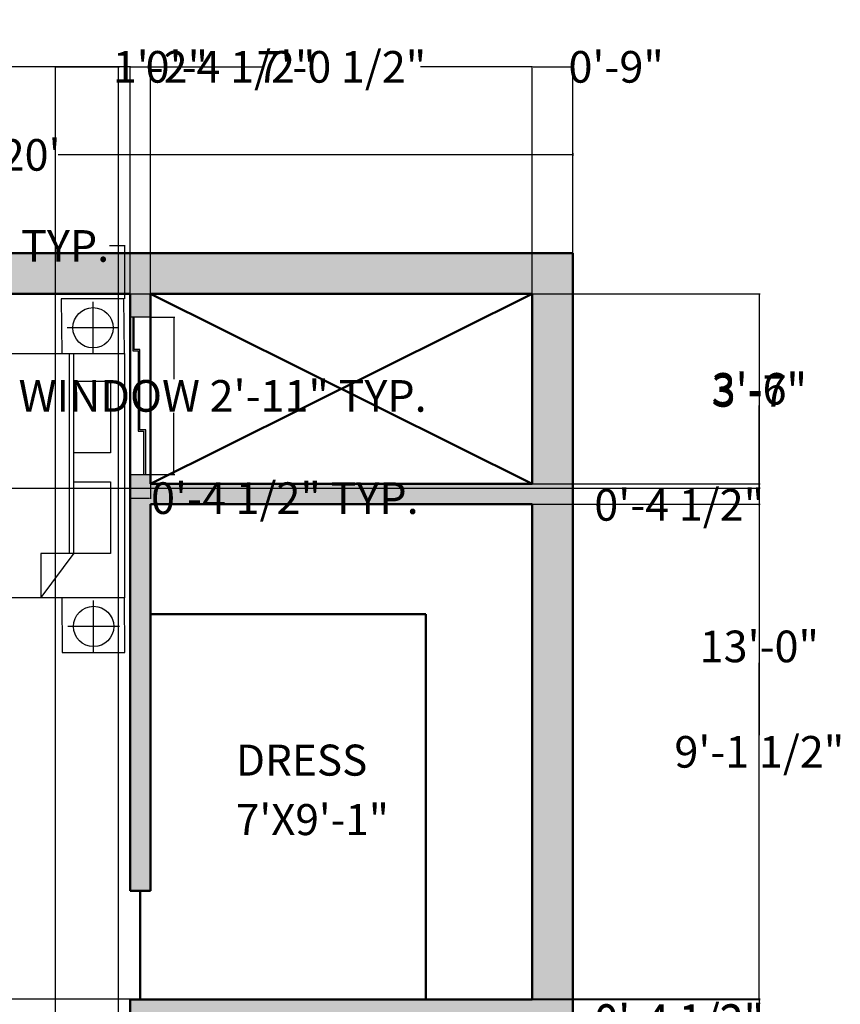
# Model space of a CAD drawing. Units: inches. Extents: x 48 to 822, y -191 to 651.
# Tile 13 of 13: x 626 to 808, y 433 to 651. Entities that reach past the tile are written whole.
import ezdxf

# ---------------------------------------------------------------- set-up
doc = ezdxf.new("R2010")
doc.units = ezdxf.units.IN
doc.header["$MEASUREMENT"] = 0
doc.layers.get('0').update_dxf_attribs({"color": 254})
for name, color, linetype, lineweight in [('A-ANNO-DIMS', 2, 'Continuous', 18), ('A-AREA-IDEN', 7, 'Continuous', 25), ('A-FURN', 8, 'Continuous', 18), ('A-GLAZ', 4, 'Continuous', 25), ('A-WALL', 7, 'Continuous', 50), ('A-WALL-PATT', 8, 'Continuous', 13)]:
    doc.layers.add(name, color=color, linetype=linetype, lineweight=lineweight)
doc.layers.add('furniture', color=250, linetype='Continuous')
doc.styles.get("Standard").update_dxf_attribs({"font": 'arial.ttf'})
doc.dimstyles.get("Standard").update_dxf_attribs({"dimtxt": 7, "dimasz": 0.18, "dimexe": 0.18, "dimexo": 0.0625, "dimgap": 0.09, "dimtad": 0, "dimtih": 1, "dimtoh": 1, "dimzin": 0, "dimdsep": 46, "dimlunit": 3, "dimtxsty": 'Standard', "dimcen": 0.09, "dimadec": 0, "dimazin": 0, "dimtfac": 1, "dimtofl": 0, "dimtmove": 0, "dimatfit": 3, "dimfxl": 1, "dimtolj": 1, "dimtzin": 0, "dimarcsym": 0})

# ---------------------------------------------------------------- blocks, each defined once
blk = doc.blocks.new('CARPET')
at = {"layer": 'furniture'}
for p, q in [((-51.53, -98.11), (-51.53, -55.12)), ((-51.53, -55.12), (-41.27, -55.12)), ((36, -55.12), (51.55, -55.12)), ((51.55, -55.12), (51.55, -98.11)), ((51.55, -98.11), (-51.53, -98.11))]:
    blk.add_line(p, q, dxfattribs=at)
for points, knots in [([(-53.37, -55.99), (-53.22, -55.8), (-52.9, -55.41), (-52.34, -55.8), (-51.89, -56.08), (-51.65, -55.91), (-51.53, -55.83)], [0, 0, 0, 0, 0.653278, 1.290138, 1.740457, 2.114451, 2.114451, 2.114451, 2.114451]), ([(53.37, -55.99), (53.22, -55.8), (52.9, -55.41), (52.34, -55.8), (51.89, -56.08), (51.65, -55.91), (51.53, -55.83)], [0, 0, 0, 0, 0.653278, 1.290138, 1.740457, 2.114451, 2.114451, 2.114451, 2.114451]), ([(-53.37, -57.26), (-53.22, -57.07), (-52.9, -56.67), (-52.34, -57.07), (-51.89, -57.35), (-51.65, -57.17), (-51.53, -57.1)], [0, 0, 0, 0, 0.653278, 1.290138, 1.740457, 2.114451, 2.114451, 2.114451, 2.114451]), ([(-53.37, -58.59), (-53.22, -58.4), (-52.9, -58.01), (-52.34, -58.4), (-51.89, -58.68), (-51.65, -58.5), (-51.53, -58.43)], [0, 0, 0, 0, 0.653278, 1.290138, 1.740457, 2.114451, 2.114451, 2.114451, 2.114451]), ([(53.37, -57.26), (53.22, -57.07), (52.9, -56.67), (52.34, -57.07), (51.89, -57.35), (51.65, -57.17), (51.53, -57.1)], [0, 0, 0, 0, 0.653278, 1.290138, 1.740457, 2.114451, 2.114451, 2.114451, 2.114451]), ([(53.37, -58.59), (53.22, -58.4), (52.9, -58.01), (52.34, -58.4), (51.89, -58.68), (51.65, -58.5), (51.53, -58.43)], [0, 0, 0, 0, 0.653278, 1.290138, 1.740457, 2.114451, 2.114451, 2.114451, 2.114451]), ([(-53.37, -59.78), (-53.22, -59.58), (-52.9, -59.19), (-52.34, -59.58), (-51.89, -59.86), (-51.65, -59.69), (-51.53, -59.61)], [0, 0, 0, 0, 0.653278, 1.290138, 1.740457, 2.114451, 2.114451, 2.114451, 2.114451]), ([(-53.37, -61.22), (-53.22, -61.02), (-52.9, -60.63), (-52.34, -61.02), (-51.89, -61.3), (-51.65, -61.13), (-51.53, -61.05)], [0, 0, 0, 0, 0.653278, 1.290138, 1.740457, 2.114451, 2.114451, 2.114451, 2.114451]), ([(-53.37, -62.44), (-53.22, -62.25), (-52.9, -61.86), (-52.34, -62.25), (-51.89, -62.53), (-51.65, -62.36), (-51.53, -62.28)], [0, 0, 0, 0, 0.653278, 1.290138, 1.740457, 2.114451, 2.114451, 2.114451, 2.114451]), ([(53.37, -59.78), (53.22, -59.58), (52.9, -59.19), (52.34, -59.58), (51.89, -59.86), (51.65, -59.69), (51.53, -59.61)], [0, 0, 0, 0, 0.653278, 1.290138, 1.740457, 2.114451, 2.114451, 2.114451, 2.114451]), ([(53.37, -61.22), (53.22, -61.02), (52.9, -60.63), (52.34, -61.02), (51.89, -61.3), (51.65, -61.13), (51.53, -61.05)], [0, 0, 0, 0, 0.653278, 1.290138, 1.740457, 2.114451, 2.114451, 2.114451, 2.114451]), ([(53.37, -62.44), (53.22, -62.25), (52.9, -61.86), (52.34, -62.25), (51.89, -62.53), (51.65, -62.36), (51.53, -62.28)], [0, 0, 0, 0, 0.653278, 1.290138, 1.740457, 2.114451, 2.114451, 2.114451, 2.114451]), ([(-53.37, -63.63), (-53.22, -63.43), (-52.9, -63.04), (-52.34, -63.43), (-51.89, -63.72), (-51.65, -63.54), (-51.53, -63.46)], [0, 0, 0, 0, 0.653278, 1.290138, 1.740457, 2.114451, 2.114451, 2.114451, 2.114451]), ([(-53.37, -65.07), (-53.22, -64.87), (-52.9, -64.48), (-52.34, -64.87), (-51.89, -65.15), (-51.65, -64.98), (-51.53, -64.9)], [0, 0, 0, 0, 0.653278, 1.290138, 1.740457, 2.114451, 2.114451, 2.114451, 2.114451]), ([(53.37, -63.63), (53.22, -63.43), (52.9, -63.04), (52.34, -63.43), (51.89, -63.72), (51.65, -63.54), (51.53, -63.46)], [0, 0, 0, 0, 0.653278, 1.290138, 1.740457, 2.114451, 2.114451, 2.114451, 2.114451]), ([(53.37, -65.07), (53.22, -64.87), (52.9, -64.48), (52.34, -64.87), (51.89, -65.15), (51.65, -64.98), (51.53, -64.9)], [0, 0, 0, 0, 0.653278, 1.290138, 1.740457, 2.114451, 2.114451, 2.114451, 2.114451]), ([(-53.37, -66.76), (-53.22, -66.56), (-52.9, -66.17), (-52.34, -66.56), (-51.89, -66.84), (-51.65, -66.67), (-51.53, -66.59)], [0, 0, 0, 0, 0.653278, 1.290138, 1.740457, 2.114451, 2.114451, 2.114451, 2.114451]), ([(-53.37, -68.2), (-53.22, -68), (-52.9, -67.61), (-52.34, -68), (-51.89, -68.28), (-51.65, -68.11), (-51.53, -68.03)], [0, 0, 0, 0, 0.653278, 1.290138, 1.740457, 2.114451, 2.114451, 2.114451, 2.114451]), ([(53.37, -66.76), (53.22, -66.56), (52.9, -66.17), (52.34, -66.56), (51.89, -66.84), (51.65, -66.67), (51.53, -66.59)], [0, 0, 0, 0, 0.653278, 1.290138, 1.740457, 2.114451, 2.114451, 2.114451, 2.114451]), ([(53.37, -68.2), (53.22, -68), (52.9, -67.61), (52.34, -68), (51.89, -68.28), (51.65, -68.11), (51.53, -68.03)], [0, 0, 0, 0, 0.653278, 1.290138, 1.740457, 2.114451, 2.114451, 2.114451, 2.114451]), ([(-53.37, -69.53), (-53.22, -69.33), (-52.9, -68.94), (-52.34, -69.33), (-51.89, -69.61), (-51.65, -69.44), (-51.53, -69.36)], [0, 0, 0, 0, 0.653278, 1.290138, 1.740457, 2.114451, 2.114451, 2.114451, 2.114451]), ([(-53.37, -70.79), (-53.22, -70.6), (-52.9, -70.21), (-52.34, -70.6), (-51.89, -70.88), (-51.65, -70.7), (-51.53, -70.63)], [0, 0, 0, 0, 0.653278, 1.290138, 1.740457, 2.114451, 2.114451, 2.114451, 2.114451]), ([(-53.37, -72.12), (-53.22, -71.93), (-52.9, -71.54), (-52.34, -71.93), (-51.89, -72.21), (-51.65, -72.04), (-51.53, -71.96)], [0, 0, 0, 0, 0.653278, 1.290138, 1.740457, 2.114451, 2.114451, 2.114451, 2.114451]), ([(53.37, -69.53), (53.22, -69.33), (52.9, -68.94), (52.34, -69.33), (51.89, -69.61), (51.65, -69.44), (51.53, -69.36)], [0, 0, 0, 0, 0.653278, 1.290138, 1.740457, 2.114451, 2.114451, 2.114451, 2.114451]), ([(53.37, -70.79), (53.22, -70.6), (52.9, -70.21), (52.34, -70.6), (51.89, -70.88), (51.65, -70.7), (51.53, -70.63)], [0, 0, 0, 0, 0.653278, 1.290138, 1.740457, 2.114451, 2.114451, 2.114451, 2.114451]), ([(53.37, -72.12), (53.22, -71.93), (52.9, -71.54), (52.34, -71.93), (51.89, -72.21), (51.65, -72.04), (51.53, -71.96)], [0, 0, 0, 0, 0.653278, 1.290138, 1.740457, 2.114451, 2.114451, 2.114451, 2.114451]), ([(-53.37, -73.31), (-53.22, -73.11), (-52.9, -72.72), (-52.34, -73.11), (-51.89, -73.4), (-51.65, -73.22), (-51.53, -73.14)], [0, 0, 0, 0, 0.653278, 1.290138, 1.740457, 2.114451, 2.114451, 2.114451, 2.114451]), ([(-53.37, -74.75), (-53.22, -74.55), (-52.9, -74.16), (-52.34, -74.55), (-51.89, -74.83), (-51.65, -74.66), (-51.53, -74.58)], [0, 0, 0, 0, 0.653278, 1.290138, 1.740457, 2.114451, 2.114451, 2.114451, 2.114451]), ([(53.37, -73.31), (53.22, -73.11), (52.9, -72.72), (52.34, -73.11), (51.89, -73.4), (51.65, -73.22), (51.53, -73.14)], [0, 0, 0, 0, 0.653278, 1.290138, 1.740457, 2.114451, 2.114451, 2.114451, 2.114451]), ([(53.37, -74.75), (53.22, -74.55), (52.9, -74.16), (52.34, -74.55), (51.89, -74.83), (51.65, -74.66), (51.53, -74.58)], [0, 0, 0, 0, 0.653278, 1.290138, 1.740457, 2.114451, 2.114451, 2.114451, 2.114451]), ([(-53.37, -75.98), (-53.22, -75.78), (-52.9, -75.39), (-52.34, -75.78), (-51.89, -76.06), (-51.65, -75.89), (-51.53, -75.81)], [0, 0, 0, 0, 0.653278, 1.290138, 1.740457, 2.114451, 2.114451, 2.114451, 2.114451]), ([(-53.37, -77.16), (-53.22, -76.96), (-52.9, -76.57), (-52.34, -76.96), (-51.89, -77.25), (-51.65, -77.07), (-51.53, -76.99)], [0, 0, 0, 0, 0.653278, 1.290138, 1.740457, 2.114451, 2.114451, 2.114451, 2.114451]), ([(53.37, -75.98), (53.22, -75.78), (52.9, -75.39), (52.34, -75.78), (51.89, -76.06), (51.65, -75.89), (51.53, -75.81)], [0, 0, 0, 0, 0.653278, 1.290138, 1.740457, 2.114451, 2.114451, 2.114451, 2.114451]), ([(53.37, -77.16), (53.22, -76.96), (52.9, -76.57), (52.34, -76.96), (51.89, -77.25), (51.65, -77.07), (51.53, -76.99)], [0, 0, 0, 0, 0.653278, 1.290138, 1.740457, 2.114451, 2.114451, 2.114451, 2.114451]), ([(-53.37, -78.6), (-53.22, -78.4), (-52.9, -78.01), (-52.34, -78.4), (-51.89, -78.68), (-51.65, -78.51), (-51.53, -78.43)], [0, 0, 0, 0, 0.653278, 1.290138, 1.740457, 2.114451, 2.114451, 2.114451, 2.114451]), ([(-53.37, -80.29), (-53.22, -80.09), (-52.9, -79.7), (-52.34, -80.09), (-51.89, -80.37), (-51.65, -80.2), (-51.53, -80.12)], [0, 0, 0, 0, 0.653278, 1.290138, 1.740457, 2.114451, 2.114451, 2.114451, 2.114451]), ([(53.37, -78.6), (53.22, -78.4), (52.9, -78.01), (52.34, -78.4), (51.89, -78.68), (51.65, -78.51), (51.53, -78.43)], [0, 0, 0, 0, 0.653278, 1.290138, 1.740457, 2.114451, 2.114451, 2.114451, 2.114451]), ([(53.37, -80.29), (53.22, -80.09), (52.9, -79.7), (52.34, -80.09), (51.89, -80.37), (51.65, -80.2), (51.53, -80.12)], [0, 0, 0, 0, 0.653278, 1.290138, 1.740457, 2.114451, 2.114451, 2.114451, 2.114451]), ([(-53.37, -81.73), (-53.22, -81.53), (-52.9, -81.14), (-52.34, -81.53), (-51.89, -81.81), (-51.65, -81.64), (-51.53, -81.56)], [0, 0, 0, 0, 0.653278, 1.290138, 1.740457, 2.114451, 2.114451, 2.114451, 2.114451]), ([(-53.37, -83.06), (-53.22, -82.86), (-52.9, -82.47), (-52.34, -82.86), (-51.89, -83.14), (-51.65, -82.97), (-51.53, -82.89)], [0, 0, 0, 0, 0.653278, 1.290138, 1.740457, 2.114451, 2.114451, 2.114451, 2.114451]), ([(-53.37, -84.18), (-53.22, -83.99), (-52.9, -83.6), (-52.34, -83.99), (-51.89, -84.27), (-51.65, -84.09), (-51.53, -84.02)], [0, 0, 0, 0, 0.653278, 1.290138, 1.740457, 2.114451, 2.114451, 2.114451, 2.114451]), ([(53.37, -81.73), (53.22, -81.53), (52.9, -81.14), (52.34, -81.53), (51.89, -81.81), (51.65, -81.64), (51.53, -81.56)], [0, 0, 0, 0, 0.653278, 1.290138, 1.740457, 2.114451, 2.114451, 2.114451, 2.114451]), ([(53.37, -83.06), (53.22, -82.86), (52.9, -82.47), (52.34, -82.86), (51.89, -83.14), (51.65, -82.97), (51.53, -82.89)], [0, 0, 0, 0, 0.653278, 1.290138, 1.740457, 2.114451, 2.114451, 2.114451, 2.114451]), ([(53.37, -84.18), (53.22, -83.99), (52.9, -83.6), (52.34, -83.99), (51.89, -84.27), (51.65, -84.09), (51.53, -84.02)], [0, 0, 0, 0, 0.653278, 1.290138, 1.740457, 2.114451, 2.114451, 2.114451, 2.114451]), ([(-53.37, -85.51), (-53.22, -85.32), (-52.9, -84.93), (-52.34, -85.32), (-51.89, -85.6), (-51.65, -85.42), (-51.53, -85.35)], [0, 0, 0, 0, 0.653278, 1.290138, 1.740457, 2.114451, 2.114451, 2.114451, 2.114451]), ([(-53.37, -86.7), (-53.22, -86.5), (-52.9, -86.11), (-52.34, -86.5), (-51.89, -86.78), (-51.65, -86.61), (-51.53, -86.53)], [0, 0, 0, 0, 0.653278, 1.290138, 1.740457, 2.114451, 2.114451, 2.114451, 2.114451]), ([(53.37, -85.51), (53.22, -85.32), (52.9, -84.93), (52.34, -85.32), (51.89, -85.6), (51.65, -85.42), (51.53, -85.35)], [0, 0, 0, 0, 0.653278, 1.290138, 1.740457, 2.114451, 2.114451, 2.114451, 2.114451]), ([(53.37, -86.7), (53.22, -86.5), (52.9, -86.11), (52.34, -86.5), (51.89, -86.78), (51.65, -86.61), (51.53, -86.53)], [0, 0, 0, 0, 0.653278, 1.290138, 1.740457, 2.114451, 2.114451, 2.114451, 2.114451]), ([(-53.37, -88.14), (-53.22, -87.94), (-52.9, -87.55), (-52.34, -87.94), (-51.89, -88.22), (-51.65, -88.05), (-51.53, -87.97)], [0, 0, 0, 0, 0.653278, 1.290138, 1.740457, 2.114451, 2.114451, 2.114451, 2.114451]), ([(-53.37, -89.36), (-53.22, -89.17), (-52.9, -88.78), (-52.34, -89.17), (-51.89, -89.45), (-51.65, -89.28), (-51.53, -89.2)], [0, 0, 0, 0, 0.653278, 1.290138, 1.740457, 2.114451, 2.114451, 2.114451, 2.114451]), ([(-53.37, -90.55), (-53.22, -90.35), (-52.9, -89.96), (-52.34, -90.35), (-51.89, -90.64), (-51.65, -90.46), (-51.53, -90.38)], [0, 0, 0, 0, 0.653278, 1.290138, 1.740457, 2.114451, 2.114451, 2.114451, 2.114451]), ([(53.37, -88.14), (53.22, -87.94), (52.9, -87.55), (52.34, -87.94), (51.89, -88.22), (51.65, -88.05), (51.53, -87.97)], [0, 0, 0, 0, 0.653278, 1.290138, 1.740457, 2.114451, 2.114451, 2.114451, 2.114451]), ([(53.37, -89.36), (53.22, -89.17), (52.9, -88.78), (52.34, -89.17), (51.89, -89.45), (51.65, -89.28), (51.53, -89.2)], [0, 0, 0, 0, 0.653278, 1.290138, 1.740457, 2.114451, 2.114451, 2.114451, 2.114451]), ([(53.37, -90.55), (53.22, -90.35), (52.9, -89.96), (52.34, -90.35), (51.9, -90.63), (51.66, -90.47), (51.55, -90.4)], [0, 0, 0, 0, 0.653278, 1.290138, 1.740457, 2.0926, 2.0926, 2.0926, 2.0926]), ([(-53.37, -91.99), (-53.22, -91.79), (-52.9, -91.4), (-52.34, -91.79), (-51.89, -92.07), (-51.65, -91.9), (-51.53, -91.82)], [0, 0, 0, 0, 0.653278, 1.290138, 1.740457, 2.114451, 2.114451, 2.114451, 2.114451]), ([(-53.37, -92.69), (-53.22, -92.48), (-52.9, -92.08), (-52.35, -92.49), (-51.89, -92.77), (-51.65, -92.6), (-51.53, -92.52)], [0, 0, 0, 0, 0.663904, 1.307406, 1.757725, 2.131719, 2.131719, 2.131719, 2.131719]), ([(-53.37, -93.61), (-53.22, -93.42), (-52.9, -93.03), (-52.34, -93.42), (-51.89, -93.7), (-51.65, -93.52), (-51.53, -93.45)], [0, 0, 0, 0, 0.653278, 1.290138, 1.740457, 2.114451, 2.114451, 2.114451, 2.114451]), ([(53.37, -91.99), (53.22, -91.79), (52.9, -91.4), (52.34, -91.79), (51.9, -92.07), (51.66, -91.91), (51.55, -91.83)], [0, 0, 0, 0, 0.653278, 1.290138, 1.740457, 2.0926, 2.0926, 2.0926, 2.0926]), ([(53.37, -92.69), (53.22, -92.49), (52.9, -92.09), (52.34, -92.49), (51.9, -92.77), (51.66, -92.61), (51.55, -92.53)], [0, 0, 0, 0, 0.656792, 1.295826, 1.746145, 2.098292, 2.098292, 2.098292, 2.098292]), ([(53.37, -93.66), (53.22, -93.46), (52.9, -93.07), (52.34, -93.46), (51.9, -93.74), (51.66, -93.58), (51.55, -93.5)], [0, 0, 0, 0, 0.653278, 1.290138, 1.740457, 2.0926, 2.0926, 2.0926, 2.0926]), ([(-53.37, -94.55), (-53.22, -94.35), (-52.9, -93.96), (-52.34, -94.35), (-51.89, -94.63), (-51.65, -94.46), (-51.53, -94.38)], [0, 0, 0, 0, 0.653278, 1.290138, 1.740457, 2.114451, 2.114451, 2.114451, 2.114451]), ([(-53.37, -95.05), (-53.22, -94.85), (-52.9, -94.46), (-52.34, -94.85), (-51.89, -95.14), (-51.65, -94.96), (-51.53, -94.88)], [0, 0, 0, 0, 0.653278, 1.290138, 1.740457, 2.114451, 2.114451, 2.114451, 2.114451]), ([(-53.37, -95.73), (-53.22, -95.54), (-52.9, -95.15), (-52.34, -95.54), (-51.89, -95.82), (-51.65, -95.65), (-51.53, -95.57)], [0, 0, 0, 0, 0.653278, 1.290138, 1.740457, 2.114451, 2.114451, 2.114451, 2.114451]), ([(-53.37, -96.38), (-53.22, -96.18), (-52.9, -95.79), (-52.34, -96.18), (-51.89, -96.47), (-51.65, -96.29), (-51.53, -96.21)], [0, 0, 0, 0, 0.653278, 1.290138, 1.740457, 2.114451, 2.114451, 2.114451, 2.114451]), ([(53.37, -95.78), (53.22, -95.58), (52.9, -95.19), (52.34, -95.58), (51.89, -95.86), (51.65, -95.69), (51.53, -95.61)], [0, 0, 0, 0, 0.653278, 1.290138, 1.740457, 2.114451, 2.114451, 2.114451, 2.114451]), ([(53.37, -96.43), (53.22, -96.23), (52.9, -95.84), (52.34, -96.23), (51.89, -96.51), (51.65, -96.34), (51.53, -96.26)], [0, 0, 0, 0, 0.653278, 1.290138, 1.740457, 2.114451, 2.114451, 2.114451, 2.114451]), ([(53.37, -94.59), (53.22, -94.4), (52.9, -94.01), (52.34, -94.4), (51.9, -94.68), (51.66, -94.51), (51.55, -94.44)], [0, 0, 0, 0, 0.653278, 1.290138, 1.740457, 2.0926, 2.0926, 2.0926, 2.0926]), ([(53.37, -95.1), (53.22, -94.9), (52.9, -94.51), (52.34, -94.9), (51.9, -95.18), (51.66, -95.02), (51.55, -94.94)], [0, 0, 0, 0, 0.653278, 1.290138, 1.740457, 2.0926, 2.0926, 2.0926, 2.0926]), ([(-53.37, -97.17), (-53.22, -96.98), (-52.9, -96.59), (-52.34, -96.98), (-51.89, -97.26), (-51.65, -97.08), (-51.53, -97.01)], [0, 0, 0, 0, 0.653278, 1.290138, 1.740457, 2.114451, 2.114451, 2.114451, 2.114451]), ([(-53.37, -97.99), (-53.22, -97.79), (-52.9, -97.4), (-52.34, -97.79), (-51.89, -98.08), (-51.65, -97.9), (-51.53, -97.82)], [0, 0, 0, 0, 0.653278, 1.290138, 1.740457, 2.114451, 2.114451, 2.114451, 2.114451]), ([(53.37, -97.22), (53.22, -97.02), (52.9, -96.63), (52.34, -97.02), (51.89, -97.3), (51.65, -97.13), (51.53, -97.05)], [0, 0, 0, 0, 0.653278, 1.290138, 1.740457, 2.114451, 2.114451, 2.114451, 2.114451]), ([(53.37, -97.99), (53.22, -97.79), (52.9, -97.4), (52.34, -97.79), (51.89, -98.08), (51.65, -97.9), (51.53, -97.82)], [0, 0, 0, 0, 0.653278, 1.290138, 1.740457, 2.114451, 2.114451, 2.114451, 2.114451])]:
    blk.add_open_spline(points, degree=3, knots=knots, dxfattribs=at)
blk = doc.blocks.new('A$C58D270C6')
at = {"layer": 'furniture'}
for p, q in [((9.09, 124.13), (9.09, 108.87)), ((1.46, 116.5), (16.73, 116.5)), ((14.97, 94.84), (24.62, 107.92)), ((24.62, 94.93), (24.62, 107.92)), ((42.08, 108), (42.08, 36)), ((14.97, 94.93), (24.62, 94.93)), ((14.97, 94.84), (14.97, 36)), ((16.22, 94.93), (16.22, 36)), ((9.25, 36), (9.25, 20.74)), ((1.62, 28.37), (16.88, 28.37))]:
    blk.add_line(p, q, dxfattribs=at)
for points in [[(18.5, 108), (18.34, 124.13), (-0.16, 124.13), (0, 108)], [(0, 108), (77.91, 108), (77.91, 36), (0, 36)], [(4.09, 94.93), (14.97, 94.93), (14.97, 73.83), (4.09, 73.83)], [(4.09, 65.23), (14.97, 65.23), (14.97, 44.13), (4.09, 44.13)], [(18.65, 19.87), (18.5, 36), (0, 36), (0.16, 19.87)]]:
    blk.add_lwpolyline(points, close=True, dxfattribs=at)
for centre in [(9.09, 116.5), (9.25, 28.37)]:
    blk.add_circle(centre, 5.95, dxfattribs=at)
at = {"layer": 'furniture', "xscale": 0.9312884925094044, "yscale": 0.9312884925094044, "zscale": 0.9312884925094044, "rotation": 90}
blk.add_blockref('CARPET', (3.79, 74.47), dxfattribs=at)
blk = doc.blocks.new('*D18')
at = {"layer": 'A-ANNO-DIMS', "color": 0, "lineweight": -2, "transparency": 16777216}
for p, q in [((508.61, 621.85), (508.61, 621.28)), ((508.79, 621.46), (622.52, 621.46)), ((748.43, 621.46), (634.7, 621.46)), ((748.61, 621.85), (748.61, 621.28))]:
    blk.add_line(p, q, dxfattribs=at)
at = {"layer": 'A-ANNO-DIMS', "color": 0, "transparency": 16777216}
for points in [[(508.79, 621.49), (508.79, 621.43), (508.61, 621.46)], [(748.43, 621.49), (748.43, 621.43), (748.61, 621.46)]]:
    blk.add_solid(points, dxfattribs=at)
at = {"layer": 'Defpoints', "color": 0, "transparency": 16777216}
for p in [(508.61, 621.91), (748.61, 621.91), (748.61, 621.46)]:
    blk.add_point(p, dxfattribs=at)
at = {"layer": 'A-ANNO-DIMS', "color": 0, "transparency": 16777216, "insert": (628.61, 621.46), "char_height": 7, "attachment_point": 5}
blk.add_mtext("\\A1;20'", dxfattribs=at)
blk = doc.blocks.new('WIN-900-SLIT')
for p, q in [((271.95, 585.52), (267.45, 585.52)), ((267.45, 585.52), (267.45, 550.72)), ((268.05, 585.52), (268.05, 578.13)), ((268.38, 578.41), (268.38, 585.52)), ((271.95, 550.72), (271.95, 585.52)), ((268.05, 578.13), (269.28, 578.13)), ((269.63, 578.41), (268.38, 578.41)), ((269.28, 578.13), (269.28, 560.35)), ((269.63, 560.61), (269.63, 578.41)), ((269.28, 560.35), (270.46, 560.35)), ((270.92, 560.61), (269.63, 560.61)), ((270.46, 560.35), (270.46, 550.72)), ((270.92, 550.72), (270.92, 560.61)), ((267.45, 550.72), (271.95, 550.72))]:
    blk.add_line(p, q)
blk = doc.blocks.new('*D41')
at = {"layer": 'A-ANNO-DIMS', "color": 0, "lineweight": -2, "transparency": 16777216}
for p, q in [((578, 589.63), (578, 601.49)), ((649.48, 589.63), (649.48, 601.49)), ((578.18, 601.31), (581.44, 601.31)), ((649.3, 601.31), (646.04, 601.31))]:
    blk.add_line(p, q, dxfattribs=at)
at = {"layer": 'A-ANNO-DIMS', "color": 0, "transparency": 16777216}
for points in [[(578.18, 601.34), (578.18, 601.28), (578, 601.31)], [(649.3, 601.34), (649.3, 601.28), (649.48, 601.31)]]:
    blk.add_solid(points, dxfattribs=at)
at = {"layer": 'Defpoints', "color": 0, "transparency": 16777216}
for p in [(578, 601.31), (578, 589.57), (649.48, 589.57)]:
    blk.add_point(p, dxfattribs=at)
at = {"layer": 'A-ANNO-DIMS', "color": 0, "transparency": 16777216, "insert": (613.74, 601.31), "char_height": 7, "attachment_point": 5}
blk.add_mtext('\\A1;5\'-11 1/2" TYP.', dxfattribs=at)
blk = doc.blocks.new('*D50')
at = {"layer": 'A-ANNO-DIMS', "color": 0, "lineweight": -2, "transparency": 16777216}
for p, q in [((655.17, 585.52), (660.51, 585.52)), ((660.33, 585.34), (660.33, 571.83)), ((660.33, 550.9), (660.33, 564.41)), ((655.17, 550.72), (660.51, 550.72))]:
    blk.add_line(p, q, dxfattribs=at)
at = {"layer": 'A-ANNO-DIMS', "color": 0, "transparency": 16777216}
for points in [[(660.3, 585.34), (660.36, 585.34), (660.33, 585.52)], [(660.3, 550.9), (660.36, 550.9), (660.33, 550.72)]]:
    blk.add_solid(points, dxfattribs=at)
at = {"layer": 'Defpoints', "color": 0, "transparency": 16777216}
for p in [(655.11, 585.52), (660.33, 585.52), (655.11, 550.72)]:
    blk.add_point(p, dxfattribs=at)
at = {"layer": 'A-ANNO-DIMS', "color": 0, "transparency": 16777216, "insert": (660.33, 568.12), "char_height": 7, "attachment_point": 5}
blk.add_mtext('\\A1;SLIT WINDOW 2\'-11" TYP.', dxfattribs=at)
blk = doc.blocks.new('*D51')
at = {"layer": 'A-ANNO-DIMS', "color": 0, "lineweight": -2, "transparency": 16777216}
for p, q in [((650.61, 550.66), (650.61, 545.32)), ((655.11, 550.66), (655.11, 545.32)), ((650.79, 545.5), (654.93, 545.5)), ((655.11, 545.5), (655.29, 545.5))]:
    blk.add_line(p, q, dxfattribs=at)
at = {"layer": 'A-ANNO-DIMS', "color": 0, "transparency": 16777216}
for points in [[(650.79, 545.53), (650.79, 545.47), (650.61, 545.5)], [(654.93, 545.53), (654.93, 545.47), (655.11, 545.5)]]:
    blk.add_solid(points, dxfattribs=at)
at = {"layer": 'Defpoints', "color": 0, "transparency": 16777216}
for p in [(650.61, 550.72), (655.11, 550.72), (655.11, 545.5)]:
    blk.add_point(p, dxfattribs=at)
at = {"layer": 'A-ANNO-DIMS', "color": 0, "transparency": 16777216, "insert": (684.87, 545.5), "char_height": 7, "attachment_point": 5}
blk.add_mtext('\\A1;0\'-4 1/2" TYP.', dxfattribs=at)
blk = doc.blocks.new('*D84')
at = {"layer": 'A-ANNO-DIMS', "color": 0, "lineweight": -2, "transparency": 16777216}
for p, q in [((356.51, 590.69), (790.04, 590.69)), ((789.86, 590.51), (789.86, 572.87)), ((789.86, 547.91), (789.86, 565.54)), ((356.51, 547.73), (790.04, 547.73))]:
    blk.add_line(p, q, dxfattribs=at)
at = {"layer": 'A-ANNO-DIMS', "color": 0, "transparency": 16777216}
for points in [[(789.83, 590.51), (789.89, 590.51), (789.86, 590.69)], [(789.83, 547.91), (789.89, 547.91), (789.86, 547.73)]]:
    blk.add_solid(points, dxfattribs=at)
at = {"layer": 'Defpoints', "color": 0, "transparency": 16777216}
for p in [(356.45, 590.69), (356.45, 547.73), (789.86, 547.73)]:
    blk.add_point(p, dxfattribs=at)
at = {"layer": 'A-ANNO-DIMS', "color": 0, "transparency": 16777216, "insert": (789.86, 569.21), "char_height": 7, "attachment_point": 5}
blk.add_mtext('\\A1;3\'-7"', dxfattribs=at)
blk = doc.blocks.new('*D97')
at = {"layer": 'A-ANNO-DIMS', "color": 0, "lineweight": -2, "transparency": 16777216}
for p, q in [((517.61, 590.75), (517.61, 641.12)), ((517.79, 640.94), (572.33, 640.94)), ((650.43, 640.94), (595.89, 640.94)), ((650.61, 590.75), (650.61, 641.12))]:
    blk.add_line(p, q, dxfattribs=at)
at = {"layer": 'A-ANNO-DIMS', "color": 0, "transparency": 16777216}
for points in [[(517.79, 640.97), (517.79, 640.91), (517.61, 640.94)], [(650.43, 640.97), (650.43, 640.91), (650.61, 640.94)]]:
    blk.add_solid(points, dxfattribs=at)
at = {"layer": 'Defpoints', "color": 0, "transparency": 16777216}
for p in [(650.61, 640.94), (517.61, 590.69), (650.61, 590.69)]:
    blk.add_point(p, dxfattribs=at)
at = {"layer": 'A-ANNO-DIMS', "color": 0, "transparency": 16777216, "insert": (584.11, 640.94), "char_height": 7, "attachment_point": 5}
blk.add_mtext('\\A1;11\'-1"', dxfattribs=at)
blk = doc.blocks.new('*D98')
at = {"layer": 'A-ANNO-DIMS', "color": 0, "lineweight": -2, "transparency": 16777216}
for p, q in [((650.61, 590.75), (650.61, 641.12)), ((650.79, 640.94), (654.93, 640.94)), ((655.11, 590.75), (655.11, 641.12)), ((655.11, 640.94), (655.29, 640.94))]:
    blk.add_line(p, q, dxfattribs=at)
at = {"layer": 'A-ANNO-DIMS', "color": 0, "transparency": 16777216}
for points in [[(650.79, 640.97), (650.79, 640.91), (650.61, 640.94)], [(654.93, 640.97), (654.93, 640.91), (655.11, 640.94)]]:
    blk.add_solid(points, dxfattribs=at)
at = {"layer": 'Defpoints', "color": 0, "transparency": 16777216}
for p in [(655.11, 640.94), (650.61, 590.69), (655.11, 590.69)]:
    blk.add_point(p, dxfattribs=at)
at = {"layer": 'A-ANNO-DIMS', "color": 0, "transparency": 16777216, "insert": (672.84, 640.94), "char_height": 7, "attachment_point": 5}
blk.add_mtext('\\A1;0\'-4 1/2"', dxfattribs=at)
blk = doc.blocks.new('*D99')
at = {"layer": 'A-ANNO-DIMS', "color": 0, "lineweight": -2, "transparency": 16777216}
for p, q in [((655.11, 590.75), (655.11, 641.12)), ((655.29, 640.94), (679.84, 640.94)), ((739.43, 640.94), (714.88, 640.94)), ((739.61, 590.75), (739.61, 641.12))]:
    blk.add_line(p, q, dxfattribs=at)
at = {"layer": 'A-ANNO-DIMS', "color": 0, "transparency": 16777216}
for points in [[(655.29, 640.97), (655.29, 640.91), (655.11, 640.94)], [(739.43, 640.97), (739.43, 640.91), (739.61, 640.94)]]:
    blk.add_solid(points, dxfattribs=at)
at = {"layer": 'Defpoints', "color": 0, "transparency": 16777216}
for p in [(739.61, 640.94), (655.11, 590.69), (739.61, 590.69)]:
    blk.add_point(p, dxfattribs=at)
at = {"layer": 'A-ANNO-DIMS', "color": 0, "transparency": 16777216, "insert": (697.36, 640.94), "char_height": 7, "attachment_point": 5}
blk.add_mtext('\\A1;7\'-0 1/2"', dxfattribs=at)
blk = doc.blocks.new('*D100')
at = {"layer": 'A-ANNO-DIMS', "color": 0, "lineweight": -2, "transparency": 16777216}
for p, q in [((739.61, 590.75), (739.61, 641.12)), ((739.79, 640.94), (748.43, 640.94)), ((748.61, 599.75), (748.61, 641.12)), ((748.61, 640.94), (748.79, 640.94))]:
    blk.add_line(p, q, dxfattribs=at)
at = {"layer": 'A-ANNO-DIMS', "color": 0, "transparency": 16777216}
for points in [[(739.79, 640.97), (739.79, 640.91), (739.61, 640.94)], [(748.43, 640.97), (748.43, 640.91), (748.61, 640.94)]]:
    blk.add_solid(points, dxfattribs=at)
at = {"layer": 'Defpoints', "color": 0, "transparency": 16777216}
for p in [(748.61, 640.94), (748.61, 599.69), (739.61, 590.69)]:
    blk.add_point(p, dxfattribs=at)
at = {"layer": 'A-ANNO-DIMS', "color": 0, "transparency": 16777216, "insert": (758.18, 640.94), "char_height": 7, "attachment_point": 5}
blk.add_mtext('\\A1;0\'-9"', dxfattribs=at)
blk = doc.blocks.new('*D105')
at = {"layer": 'A-ANNO-DIMS', "color": 0, "lineweight": -2, "transparency": 16777216}
for p, q in [((517.67, 590.69), (790.04, 590.69)), ((789.86, 590.51), (789.86, 516.35)), ((789.86, 434.87), (789.86, 509.02)), ((517.67, 434.69), (790.04, 434.69))]:
    blk.add_line(p, q, dxfattribs=at)
at = {"layer": 'A-ANNO-DIMS', "color": 0, "transparency": 16777216}
for points in [[(789.83, 590.51), (789.89, 590.51), (789.86, 590.69)], [(789.83, 434.87), (789.89, 434.87), (789.86, 434.69)]]:
    blk.add_solid(points, dxfattribs=at)
at = {"layer": 'Defpoints', "color": 0, "transparency": 16777216}
for p in [(517.61, 590.69), (517.61, 434.69), (789.86, 434.69)]:
    blk.add_point(p, dxfattribs=at)
at = {"layer": 'A-ANNO-DIMS', "color": 0, "transparency": 16777216, "insert": (789.86, 512.69), "char_height": 7, "attachment_point": 5}
blk.add_mtext('\\A1;13\'-0"', dxfattribs=at)
blk = doc.blocks.new('*D106')
at = {"layer": 'A-ANNO-DIMS', "color": 0, "lineweight": -2, "transparency": 16777216}
for p, q in [((517.67, 434.69), (790.04, 434.69)), ((789.86, 434.51), (789.86, 430.37)), ((517.67, 430.19), (790.04, 430.19)), ((789.86, 430.01), (789.68, 430.01)), ((789.86, 430.19), (789.86, 430.01))]:
    blk.add_line(p, q, dxfattribs=at)
at = {"layer": 'A-ANNO-DIMS', "color": 0, "transparency": 16777216}
for points in [[(789.83, 434.51), (789.89, 434.51), (789.86, 434.69)], [(789.83, 430.37), (789.89, 430.37), (789.86, 430.19)]]:
    blk.add_solid(points, dxfattribs=at)
at = {"layer": 'Defpoints', "color": 0, "transparency": 16777216}
for p in [(517.61, 434.69), (517.61, 430.19), (789.86, 430.19)]:
    blk.add_point(p, dxfattribs=at)
at = {"layer": 'A-ANNO-DIMS', "color": 0, "transparency": 16777216, "insert": (772.13, 430.01), "char_height": 7, "attachment_point": 5}
blk.add_mtext('\\A1;0\'-4 1/2"', dxfattribs=at)
blk = doc.blocks.new('*D118')
at = {"layer": 'A-ANNO-DIMS', "color": 0, "lineweight": -2, "transparency": 16777216}
for p, q in [((739.67, 590.69), (790.04, 590.69)), ((789.86, 590.51), (789.86, 573.35)), ((789.86, 548.87), (789.86, 566.02)), ((739.67, 548.69), (790.04, 548.69))]:
    blk.add_line(p, q, dxfattribs=at)
at = {"layer": 'A-ANNO-DIMS', "color": 0, "transparency": 16777216}
for points in [[(789.83, 590.51), (789.89, 590.51), (789.86, 590.69)], [(789.83, 548.87), (789.89, 548.87), (789.86, 548.69)]]:
    blk.add_solid(points, dxfattribs=at)
at = {"layer": 'Defpoints', "color": 0, "transparency": 16777216}
for p in [(739.61, 590.69), (739.61, 548.69), (789.86, 548.69)]:
    blk.add_point(p, dxfattribs=at)
at = {"layer": 'A-ANNO-DIMS', "color": 0, "transparency": 16777216, "insert": (789.86, 569.69), "char_height": 7, "attachment_point": 5}
blk.add_mtext('\\A1;3\'-6"', dxfattribs=at)
blk = doc.blocks.new('*D119')
at = {"layer": 'A-ANNO-DIMS', "color": 0, "lineweight": -2, "transparency": 16777216}
for p, q in [((739.67, 548.69), (790.04, 548.69)), ((789.86, 548.51), (789.86, 544.37)), ((739.67, 544.19), (790.04, 544.19)), ((789.86, 544.01), (789.68, 544.01)), ((789.86, 544.19), (789.86, 544.01))]:
    blk.add_line(p, q, dxfattribs=at)
at = {"layer": 'A-ANNO-DIMS', "color": 0, "transparency": 16777216}
for points in [[(789.83, 548.51), (789.89, 548.51), (789.86, 548.69)], [(789.83, 544.37), (789.89, 544.37), (789.86, 544.19)]]:
    blk.add_solid(points, dxfattribs=at)
at = {"layer": 'Defpoints', "color": 0, "transparency": 16777216}
for p in [(739.61, 548.69), (739.61, 544.19), (789.86, 544.19)]:
    blk.add_point(p, dxfattribs=at)
at = {"layer": 'A-ANNO-DIMS', "color": 0, "transparency": 16777216, "insert": (772.13, 544.01), "char_height": 7, "attachment_point": 5}
blk.add_mtext('\\A1;0\'-4 1/2"', dxfattribs=at)
blk = doc.blocks.new('*D120')
at = {"layer": 'A-ANNO-DIMS', "color": 0, "lineweight": -2, "transparency": 16777216}
for p, q in [((739.67, 544.19), (790.04, 544.19)), ((789.86, 544.01), (789.86, 493.07)), ((789.86, 434.72), (789.86, 485.65)), ((739.67, 434.54), (790.04, 434.54))]:
    blk.add_line(p, q, dxfattribs=at)
at = {"layer": 'A-ANNO-DIMS', "color": 0, "transparency": 16777216}
for points in [[(789.83, 544.01), (789.89, 544.01), (789.86, 544.19)], [(789.83, 434.72), (789.89, 434.72), (789.86, 434.54)]]:
    blk.add_solid(points, dxfattribs=at)
at = {"layer": 'Defpoints', "color": 0, "transparency": 16777216}
for p in [(739.61, 544.19), (739.61, 434.54), (789.86, 434.54)]:
    blk.add_point(p, dxfattribs=at)
at = {"layer": 'A-ANNO-DIMS', "color": 0, "transparency": 16777216, "insert": (789.86, 489.36), "char_height": 7, "attachment_point": 5}
blk.add_mtext('\\A1;9\'-1 1/2"', dxfattribs=at)
blk = doc.blocks.new('*D121')
at = {"layer": 'A-ANNO-DIMS', "color": 0, "lineweight": -2, "transparency": 16777216}
for p, q in [((739.67, 434.54), (790.04, 434.54)), ((789.86, 434.36), (789.86, 430.22)), ((739.67, 430.04), (790.04, 430.04)), ((789.86, 429.86), (789.68, 429.86)), ((789.86, 430.04), (789.86, 429.86))]:
    blk.add_line(p, q, dxfattribs=at)
at = {"layer": 'A-ANNO-DIMS', "color": 0, "transparency": 16777216}
for points in [[(789.83, 434.36), (789.89, 434.36), (789.86, 434.54)], [(789.83, 430.22), (789.89, 430.22), (789.86, 430.04)]]:
    blk.add_solid(points, dxfattribs=at)
at = {"layer": 'Defpoints', "color": 0, "transparency": 16777216}
for p in [(739.61, 434.54), (739.61, 430.04), (789.86, 430.04)]:
    blk.add_point(p, dxfattribs=at)
at = {"layer": 'A-ANNO-DIMS', "color": 0, "transparency": 16777216, "insert": (772.13, 429.86), "char_height": 7, "attachment_point": 5}
blk.add_mtext('\\A1;0\'-4 1/2"', dxfattribs=at)
blk = doc.blocks.new('*D125')
at = {"layer": 'A-ANNO-DIMS', "color": 0, "lineweight": -2, "transparency": 16777216}
for p, q in [((634.1, 295.25), (634.1, 641.12)), ((634.28, 640.94), (647.91, 640.94)), ((648.09, 295.25), (648.09, 641.12)), ((648.09, 640.94), (648.27, 640.94))]:
    blk.add_line(p, q, dxfattribs=at)
at = {"layer": 'A-ANNO-DIMS', "color": 0, "transparency": 16777216}
for points in [[(634.28, 640.97), (634.28, 640.91), (634.1, 640.94)], [(647.91, 640.97), (647.91, 640.91), (648.09, 640.94)]]:
    blk.add_solid(points, dxfattribs=at)
at = {"layer": 'Defpoints', "color": 0, "transparency": 16777216}
for p in [(648.09, 640.94), (634.1, 295.19), (648.09, 295.19)]:
    blk.add_point(p, dxfattribs=at)
at = {"layer": 'A-ANNO-DIMS', "color": 0, "transparency": 16777216, "insert": (657.33, 640.94), "char_height": 7, "attachment_point": 5}
blk.add_mtext('\\A1;1\'-2"', dxfattribs=at)
blk = doc.blocks.new('*D126')
at = {"layer": 'A-ANNO-DIMS', "color": 0, "lineweight": -2, "transparency": 16777216}
for p, q in [((553.61, 295.25), (553.61, 641.12)), ((553.79, 640.94), (580.61, 640.94)), ((647.91, 640.94), (621.09, 640.94)), ((648.09, 295.25), (648.09, 641.12))]:
    blk.add_line(p, q, dxfattribs=at)
at = {"layer": 'A-ANNO-DIMS', "color": 0, "transparency": 16777216}
for points in [[(553.79, 640.97), (553.79, 640.91), (553.61, 640.94)], [(647.91, 640.97), (647.91, 640.91), (648.09, 640.94)]]:
    blk.add_solid(points, dxfattribs=at)
at = {"layer": 'Defpoints', "color": 0, "transparency": 16777216}
for p in [(648.09, 640.94), (553.61, 295.19), (648.09, 295.19)]:
    blk.add_point(p, dxfattribs=at)
at = {"layer": 'A-ANNO-DIMS', "color": 0, "transparency": 16777216, "insert": (600.85, 640.94), "char_height": 7, "attachment_point": 5}
blk.add_mtext('\\A1;7\'-10 1/2"', dxfattribs=at)

msp = doc.modelspace()

# ---------------------------------------------------------------- hatches: boundary and pattern name
at = {"layer": 'A-WALL-PATT'}
h = msp.add_hatch(color=256, dxfattribs=at)
h.dxf.hatch_style = 1
h.paths.add_polyline_path([(614.11, 432.437), (609.61, 432.437), (609.61, 376.187), (535.284, 376.187), (535.284, 371.687), (547.61, 371.687), (547.61, 359.12), (552.11, 359.12), (552.11, 371.687), (609.61, 371.687), (609.61, 335.687), (614.11, 335.687)], flags=17)
h.paths.add_polyline_path([(614.11, 434.687), (609.61, 434.687), (609.61, 432.437), (614.11, 432.437)], flags=17)
h.paths.add_polyline_path([(573.934, 434.687), (517.61, 434.687), (517.61, 590.687), (650.61, 590.687), (650.61, 585.522), (655.11, 585.522), (655.11, 590.687), (739.61, 590.687), (739.61, 548.687), (655.11, 548.687), (655.11, 550.72), (650.61, 550.72), (650.61, 458.608), (655.11, 458.608), (655.11, 544.187), (739.61, 544.187), (739.61, 434.541), (650.61, 434.541), (650.61, 430.041), (739.61, 430.041), (739.61, -16.844), (729.973, -16.844), (729.973, -21.344), (748.61, -21.344), (748.61, 599.687), (508.61, 599.687), (508.61, -120.313), (543.114, -120.313), (543.114, -111.313), (517.61, -111.313), (517.61, 38.687), (607.29, 38.687), (607.29, 43.187), (517.61, 43.187), (517.61, 97.187), (654.61, 97.187), (654.61, 30.562), (659.11, 30.562), (659.11, 101.895), (654.61, 101.895), (654.61, 101.687), (517.61, 101.687), (517.61, 221.687), (654.61, 221.687), (654.61, 218.066), (659.11, 218.066), (659.11, 226.187), (517.61, 226.187), (517.61, 295.187), (614.11, 295.187), (648.087, 295.187), (661.07, 295.187), (661.07, 299.687), (614.11, 299.687), (552.11, 299.687), (552.11, 341.37), (547.61, 341.37), (547.61, 299.687), (517.61, 299.687), (517.61, 371.687), (517.534, 371.687), (517.534, 376.187), (517.61, 430.187), (573.934, 430.187)])
h.paths.add_polyline_path([(659.11, -87.328), (654.61, -87.328), (654.61, -111.313), (598.94, -111.313), (598.94, -120.313), (659.11, -120.313)], flags=0)
h.paths.add_polyline_path([(671.266, -16.844), (659.11, -16.844), (659.11, -12.05), (654.61, -12.05), (654.61, -31.502), (659.11, -31.502), (659.11, -21.344), (671.266, -21.344)], flags=17)
h.paths.add_polyline_path([(606.11, 97.187), (601.61, 97.187), (601.61, 75.902), (606.11, 75.902)], flags=17)
h.paths.add_polyline_path([(659.11, 169.875), (654.61, 169.875), (654.61, 157.721), (659.11, 157.721)], flags=17)
h = msp.add_hatch(color=256, dxfattribs=at)
h.dxf.hatch_style = 1
h.paths.add_polyline_path([(268.379, 585.522), (268.046, 585.522), (268.046, 578.127), (269.281, 578.127), (269.281, 560.346), (270.462, 560.346), (270.462, 550.72), (270.919, 550.72), (270.919, 560.611), (269.63, 560.611), (269.63, 578.406), (268.379, 578.406)])
h.paths.add_polyline_path([(315.954, 546.588), (346.307, 546.588), (346.307, 547.726), (356.451, 547.726), (356.451, 548.166), (345.839, 548.166), (345.839, 547.241), (315.513, 547.241), (315.513, 546.437), (300.625, 546.437), (300.625, 545.795), (315.954, 545.795)])
h.paths.add_polyline_path([(651.539, 585.522), (651.206, 585.522), (651.206, 578.127), (652.441, 578.127), (652.441, 560.346), (653.621, 560.346), (653.621, 550.72), (654.078, 550.72), (654.078, 560.611), (652.789, 560.611), (652.789, 578.406), (651.539, 578.406)])
h.paths.add_polyline_path([(656.709, 147.578), (655.571, 147.578), (655.571, 157.721), (655.131, 157.721), (655.131, 147.109), (656.055, 147.109), (656.055, 116.783), (656.86, 116.783), (656.86, 101.895), (657.501, 101.895), (657.501, 117.224), (656.709, 117.224)])

# ---------------------------------------------------------------- linework, layer by layer
at = {"layer": 'A-WALL'}
for p, q in [((508.61, 599.687), (748.61, 599.687)), ((748.61, 599.687), (748.61, -120.313)), ((517.61, 590.687), (650.61, 590.687)), ((650.61, 458.608), (650.61, 590.687)), ((655.11, 548.687), (655.11, 590.687)), ((655.11, 590.687), (739.61, 548.687)), ((655.11, 548.687), (739.61, 590.687)), ((655.11, 590.687), (739.61, 590.687)), ((739.61, 590.687), (739.61, 548.687)), ((655.11, 548.687), (739.61, 548.687)), ((655.11, 544.187), (739.61, 544.187)), ((655.11, 458.608), (655.11, 544.187)), ((739.61, 544.187), (739.61, 434.541)), ((655.11, 519.798), (716.097, 519.798)), ((716.097, 519.798), (716.097, 434.541)), ((650.61, 458.608), (655.11, 458.608)), ((652.86, 458.608), (652.86, 434.541)), ((650.61, 434.541), (739.61, 434.541)), ((650.61, 434.541), (650.61, 430.041))]:
    msp.add_line(p, q, dxfattribs=at)

# ---------------------------------------------------------------- block references
at = {"layer": 'A-FURN', "xscale": 0.7500000390647866, "yscale": 0.7500000390647866, "zscale": 0.7500000390647866, "rotation": 180}
msp.add_blockref('A$C58D270C6', (649.367, 604.474), dxfattribs=at)
at = {"layer": 'A-GLAZ'}
msp.add_blockref('WIN-900-SLIT', (383.16, 0), dxfattribs=at)

# ---------------------------------------------------------------- texts
at = {"layer": 'A-AREA-IDEN'}
for s, p in [('DRESS', (674.04, 484.09)), ('7\'X9\'-1"', (674.04, 470.931))]:
    msp.add_text(s, height=6.866, dxfattribs=at).set_placement(p)

# ---------------------------------------------------------------- dimensions: what is measured, and where the dimension line sits
at = {"layer": 'A-ANNO-DIMS'}
for base, p1, p2, override, picture, middle in [((648.087, 640.937), (553.61, 295.187), (648.087, 295.187), {"dimdec": 1, "dimlfac": 1, "dimrnd": 0, "dimzin": 1, "dimdsep": 46, "dimlunit": 4, "dimfrac": 2}, '*D126', (600.849, 640.937)), ((655.11, 640.937), (650.61, 590.687), (655.11, 590.687), {"dimdec": 1, "dimlfac": 1, "dimrnd": 0, "dimzin": 1, "dimdsep": 46, "dimlunit": 4, "dimfrac": 2}, '*D98', (672.84, 640.937)), ((739.61, 640.937), (655.11, 590.687), (739.61, 590.687), {"dimdec": 1, "dimlfac": 1, "dimrnd": 0, "dimzin": 1, "dimdsep": 46, "dimlunit": 4, "dimfrac": 2}, '*D99', (697.36, 640.937)), ((650.61, 640.937), (517.61, 590.687), (650.61, 590.687), {"dimdec": 1, "dimlfac": 1, "dimrnd": 0, "dimzin": 1, "dimdsep": 46, "dimlunit": 4, "dimfrac": 2}, '*D97', (584.11, 640.937)), ((648.087, 640.937), (634.101, 295.187), (648.087, 295.187), {"dimdec": 1, "dimlfac": 1, "dimrnd": 0, "dimzin": 1, "dimdsep": 46, "dimlunit": 4, "dimfrac": 2}, '*D125', (657.331, 640.937)), ((748.61, 640.937), (739.61, 590.687), (748.61, 599.687), {"dimdec": 1, "dimlfac": 1, "dimrnd": 0, "dimzin": 1, "dimdsep": 46, "dimlunit": 4, "dimfrac": 2}, '*D100', (758.184, 640.937)), ((748.61, 621.465), (508.61, 621.913), (748.61, 621.913), {"dimclrd": 0, "dimclre": 0, "dimclrt": 0}, '*D18', (628.61, 621.465))]:
    dim = msp.add_linear_dim(base=base, p1=p1, p2=p2, dimstyle='Standard', override=override, dxfattribs=at)
    dim.commit()
    dim.dimension.update_dxf_attribs({"geometry": picture, "text_midpoint": middle})
for base, p1, p2, angle, text, picture, middle in [((577.998, 601.307), (649.484, 589.572), (577.998, 589.572), 180, '<> TYP.', '*D41', (613.741, 601.307)), ((660.331, 585.522), (655.11, 550.72), (655.11, 585.522), 90, 'SLIT WINDOW <> TYP.', '*D50', (660.331, 568.121))]:
    dim = msp.add_linear_dim(base=base, p1=p1, p2=p2, angle=angle, text=text, dimstyle='Standard', override={"dimdec": 1, "dimlfac": 1, "dimrnd": 0, "dimzin": 1, "dimdsep": 46, "dimlunit": 4, "dimfrac": 2}, dxfattribs=at)
    dim.commit()
    dim.dimension.update_dxf_attribs({"geometry": picture, "text_midpoint": middle})
for base, p1, p2, picture, middle in [((789.86, 547.726), (356.451, 590.687), (356.451, 547.726), '*D84', (789.86, 569.206)), ((789.86, 434.687), (517.61, 590.687), (517.61, 434.687), '*D105', (789.86, 512.687)), ((789.86, 548.687), (739.61, 590.687), (739.61, 548.687), '*D118', (789.86, 569.687)), ((789.86, 544.187), (739.61, 548.687), (739.61, 544.187), '*D119', (772.131, 544.007)), ((789.86, 434.541), (739.61, 544.187), (739.61, 434.541), '*D120', (789.86, 489.364)), ((789.86, 430.187), (517.61, 434.687), (517.61, 430.187), '*D106', (772.131, 430.007)), ((789.86, 430.041), (739.61, 434.541), (739.61, 430.041), '*D121', (772.131, 429.861))]:
    dim = msp.add_linear_dim(base=base, p1=p1, p2=p2, angle=90, dimstyle='Standard', override={"dimdec": 1, "dimlfac": 1, "dimrnd": 0, "dimzin": 1, "dimdsep": 46, "dimlunit": 4, "dimfrac": 2}, dxfattribs=at)
    dim.commit()
    dim.dimension.update_dxf_attribs({"geometry": picture, "text_midpoint": middle})
dim = msp.add_linear_dim(base=(655.11, 545.5), p1=(650.61, 550.72), p2=(655.11, 550.72), text='<> TYP.', dimstyle='Standard', override={"dimdec": 1, "dimlfac": 1, "dimrnd": 0, "dimzin": 1, "dimdsep": 46, "dimlunit": 4, "dimfrac": 2}, dxfattribs=at)
dim.commit()
dim.dimension.update_dxf_attribs({"geometry": '*D51', "text_midpoint": (684.87, 545.5)})

doc.saveas('drawing.dxf')
